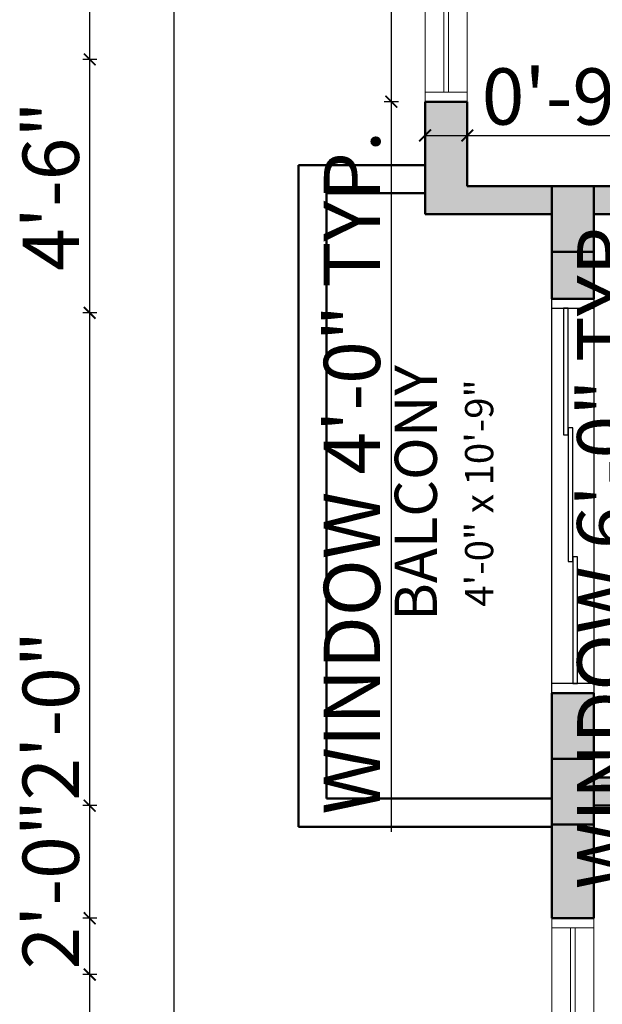
# Model space of a CAD drawing. Units: inches. Extents: x 375 to 1122, y 27 to 1069.
# Tile 72 of 155: x 385 to 509, y 667 to 877. Entities that reach past the tile are written whole.
import ezdxf

# ---------------------------------------------------------------- set-up
doc = ezdxf.new("R2010")
doc.units = ezdxf.units.IN
for name, color, linetype, lineweight in [('A-ANNO-DIMS', 2, 'Continuous', 18), ('A-AREA-IDEN', 7, 'Continuous', 18), ('A-COLS-PATT', 10, 'Continuous', 13), ('A-WALL-PATT', 252, 'Continuous', 13), ('Columns', 10, 'Continuous', 50), ('Doors', 150, 'Continuous', 25), ('Walls', 250, 'Continuous', 50), ('Windows', 122, 'Continuous', 18)]:
    doc.layers.add(name, color=color, linetype=linetype, lineweight=lineweight)
doc.styles.get("Standard").update_dxf_attribs({"font": 'arial.ttf'})
doc.dimstyles.new('ISO-25', dxfattribs={"dimtxt": 12, "dimasz": 2.5, "dimexe": 1.5, "dimexo": 1.5, "dimtad": 1, "dimdec": 1, "dimlunit": 3, "dimtxsty": 'Standard', "dimblk": 'ARCHTICK', "dimcen": 2.5, "dimadec": 0, "dimazin": 0, "dimtfac": 1, "dimtdec": 1, "dimtmove": 0, "dimatfit": 3, "dimfxl": 1.5, "dimfxlon": 1, "dimarcsym": 0})

# ---------------------------------------------------------------- blocks, each defined once
blk = doc.blocks.new('_ArchTick')
at = {"color": 0, "linetype": 'ByBlock', "const_width": 0.15}
blk.add_lwpolyline([(-0.5, -0.5), (0.5, 0.5)], dxfattribs=at)
blk = doc.blocks.new('*D28')
at = {"layer": 'A-ANNO-DIMS', "color": 0, "lineweight": -2, "transparency": 16777216}
for p, q in [((419.42, 982.53), (416.42, 982.53)), ((417.92, 982.53), (417.92, 187.53)), ((419.42, 187.53), (416.42, 187.53))]:
    blk.add_line(p, q, dxfattribs=at)
at = {"layer": 'Defpoints', "color": 0, "transparency": 16777216}
for p in [(444.51, 982.53), (417.92, 187.53), (444.51, 187.53)]:
    blk.add_point(p, dxfattribs=at)
at = {"layer": 'A-ANNO-DIMS', "color": 0, "lineweight": -2, "transparency": 16777216, "xscale": 2.5, "yscale": 2.5, "zscale": 2.5}
for p, rotation in [((417.92, 982.53), 90), ((417.92, 187.53), 270)]:
    blk.add_blockref('_ArchTick', p, dxfattribs=dict(at, rotation=rotation))
at = {"layer": 'A-ANNO-DIMS', "color": 0, "transparency": 16777216, "insert": (411.17, 585.03), "char_height": 12, "attachment_point": 5, "rotation": 90}
blk.add_mtext('66\'-3"', dxfattribs=at)
blk = doc.blocks.new('WINDOW-48IN')
for p, q in [((2, 5), (46, 5)), ((2, 4), (46, 4))]:
    blk.add_line(p, q)
blk.add_lwpolyline([(48, 0), (0, 0), (0, 9), (48, 9)], close=True)
for points in [[(2, 0), (2, 9)], [(46, 9), (46, 0)]]:
    blk.add_lwpolyline(points)
blk = doc.blocks.new('WINDOW-72IN')
for p, q in [((4, 70), (4, 2)), ((5, 70), (5, 2))]:
    blk.add_line(p, q)
blk.add_lwpolyline([(9, 0), (0, 0), (0, 72), (9, 72)], close=True)
for points in [[(0, 70), (9, 70)], [(9, 2), (0, 2)]]:
    blk.add_lwpolyline(points)
blk = doc.blocks.new('BALCONY-SLIDER-3P-84IN')
for points in [[(0, 84), (9, 84), (9, 0), (0, 0)], [(2.5, 55), (3.5, 55), (3.5, 82), (2.5, 82)], [(3.5, 28), (4.5, 28), (4.5, 56.5), (3.5, 56.5)], [(4.5, 2), (5.5, 2), (5.5, 29), (4.5, 29)]]:
    blk.add_lwpolyline(points, close=True)
for points in [[(0, 82), (9, 82)], [(9, 2), (0, 2)]]:
    blk.add_lwpolyline(points)
blk = doc.blocks.new('COLUMN-14X9IN')
blk.add_lwpolyline([(0, 0), (14, 0), (14, 9), (0, 9)], close=True)
blk = doc.blocks.new('*D47')
at = {"layer": 'A-ANNO-DIMS', "color": 0, "lineweight": -2, "transparency": 16777216}
for p, q in [((465.81, 907.53), (462.81, 907.53)), ((464.31, 907.53), (464.31, 859.53)), ((465.81, 859.53), (462.81, 859.53)), ((464.31, 859.53), (464.31, 703.93))]:
    blk.add_line(p, q, dxfattribs=at)
at = {"layer": 'Defpoints', "color": 0, "transparency": 16777216}
for p in [(471.51, 907.53), (464.31, 859.53), (471.51, 859.53)]:
    blk.add_point(p, dxfattribs=at)
at = {"layer": 'A-ANNO-DIMS', "color": 0, "lineweight": -2, "transparency": 16777216, "xscale": 2.5, "yscale": 2.5, "zscale": 2.5}
for p, rotation in [((464.31, 907.53), 90), ((464.31, 859.53), 270)]:
    blk.add_blockref('_ArchTick', p, dxfattribs=dict(at, rotation=rotation))
at = {"layer": 'A-ANNO-DIMS', "color": 0, "transparency": 16777216, "insert": (457.47, 780.48), "char_height": 12, "attachment_point": 5, "rotation": 90}
blk.add_mtext('WINDOW 4\'-0" TYP.', dxfattribs=at)
blk = doc.blocks.new('*D48')
at = {"layer": 'A-ANNO-DIMS', "color": 0, "lineweight": -2, "transparency": 16777216}
for p, q in [((471.51, 853.83), (471.51, 850.83)), ((471.51, 852.33), (480.51, 852.33)), ((480.51, 853.83), (480.51, 850.83)), ((480.51, 852.33), (557.4, 852.33))]:
    blk.add_line(p, q, dxfattribs=at)
at = {"layer": 'Defpoints', "color": 0, "transparency": 16777216}
for p in [(471.51, 859.53), (480.51, 859.53), (480.51, 852.33)]:
    blk.add_point(p, dxfattribs=at)
at = {"layer": 'A-ANNO-DIMS', "color": 0, "lineweight": -2, "transparency": 16777216, "xscale": 2.5, "yscale": 2.5, "zscale": 2.5, "rotation": 180}
blk.add_blockref('_ArchTick', (471.51, 852.33), dxfattribs=at)
at = {"layer": 'A-ANNO-DIMS', "color": 0, "lineweight": -2, "transparency": 16777216, "xscale": 2.5, "yscale": 2.5, "zscale": 2.5}
blk.add_blockref('_ArchTick', (480.51, 852.33), dxfattribs=at)
at = {"layer": 'A-ANNO-DIMS', "color": 0, "transparency": 16777216, "insert": (520.21, 859.08), "char_height": 12, "attachment_point": 5}
blk.add_mtext('0\'-9" TYP.', dxfattribs=at)
blk = doc.blocks.new('*D69')
at = {"layer": 'A-ANNO-DIMS', "color": 0, "lineweight": -2, "transparency": 16777216}
for p, q in [((518.31, 685.53), (518.31, 841.13)), ((516.81, 685.53), (519.81, 685.53)), ((518.31, 613.53), (518.31, 685.53)), ((516.81, 613.53), (519.81, 613.53))]:
    blk.add_line(p, q, dxfattribs=at)
at = {"layer": 'Defpoints', "color": 0, "transparency": 16777216}
for p in [(507.51, 685.53), (518.31, 685.53), (507.51, 613.53)]:
    blk.add_point(p, dxfattribs=at)
at = {"layer": 'A-ANNO-DIMS', "color": 0, "lineweight": -2, "transparency": 16777216, "xscale": 2.5, "yscale": 2.5, "zscale": 2.5}
for p, rotation in [((518.31, 685.53), 90), ((518.31, 613.53), 270)]:
    blk.add_blockref('_ArchTick', p, dxfattribs=dict(at, rotation=rotation))
at = {"layer": 'A-ANNO-DIMS', "color": 0, "transparency": 16777216, "insert": (511.47, 764.58), "char_height": 12, "attachment_point": 5, "rotation": 90}
blk.add_mtext('WINDOW 6\'-0" TYP.', dxfattribs=at)
blk = doc.blocks.new('*D82')
at = {"layer": 'A-ANNO-DIMS', "color": 0, "lineweight": -2, "transparency": 16777216}
for p, q in [((401.51, 1009.53), (398.51, 1009.53)), ((400.01, 160.53), (400.01, 1009.53)), ((401.51, 160.53), (398.51, 160.53))]:
    blk.add_line(p, q, dxfattribs=at)
at = {"layer": 'Defpoints', "color": 0, "transparency": 16777216}
for p in [(400.01, 1009.53), (630.53, 1009.53), (630.53, 160.53)]:
    blk.add_point(p, dxfattribs=at)
at = {"layer": 'A-ANNO-DIMS', "color": 0, "lineweight": -2, "transparency": 16777216, "xscale": 2.5, "yscale": 2.5, "zscale": 2.5}
for p, rotation in [((400.01, 1009.53), 90), ((400.01, 160.53), 270)]:
    blk.add_blockref('_ArchTick', p, dxfattribs=dict(at, rotation=rotation))
at = {"layer": 'A-ANNO-DIMS', "color": 0, "transparency": 16777216, "insert": (393.26, 585.03), "char_height": 12, "attachment_point": 5, "rotation": 90}
blk.add_mtext('70\'-9"', dxfattribs=at)
blk = doc.blocks.new('*D85')
at = {"layer": 'A-ANNO-DIMS', "color": 0, "lineweight": -2, "transparency": 16777216}
for p, q in [((401.51, 868.53), (398.51, 868.53)), ((400.01, 814.53), (400.01, 868.53)), ((401.51, 814.53), (398.51, 814.53))]:
    blk.add_line(p, q, dxfattribs=at)
at = {"layer": 'Defpoints', "color": 0, "transparency": 16777216}
for p in [(400.01, 868.53), (845.01, 868.53), (845.01, 814.53)]:
    blk.add_point(p, dxfattribs=at)
at = {"layer": 'A-ANNO-DIMS', "color": 0, "lineweight": -2, "transparency": 16777216, "xscale": 2.5, "yscale": 2.5, "zscale": 2.5}
for p, rotation in [((400.01, 868.53), 90), ((400.01, 814.53), 270)]:
    blk.add_blockref('_ArchTick', p, dxfattribs=dict(at, rotation=rotation))
at = {"layer": 'A-ANNO-DIMS', "color": 0, "transparency": 16777216, "insert": (393.26, 841.53), "char_height": 12, "attachment_point": 5, "rotation": 90}
blk.add_mtext('4\'-6"', dxfattribs=at)
blk = doc.blocks.new('*D93')
at = {"layer": 'A-ANNO-DIMS', "color": 0, "lineweight": -2, "transparency": 16777216}
for p, q in [((400.01, 673.53), (400.01, 709.38)), ((401.51, 673.53), (398.51, 673.53)), ((400.01, 649.53), (400.01, 673.53)), ((401.51, 649.53), (398.51, 649.53))]:
    blk.add_line(p, q, dxfattribs=at)
at = {"layer": 'Defpoints', "color": 0, "transparency": 16777216}
for p in [(400.01, 673.53), (663.51, 673.53), (663.51, 649.53)]:
    blk.add_point(p, dxfattribs=at)
at = {"layer": 'A-ANNO-DIMS', "color": 0, "lineweight": -2, "transparency": 16777216, "xscale": 2.5, "yscale": 2.5, "zscale": 2.5}
for p, rotation in [((400.01, 673.53), 90), ((400.01, 649.53), 270)]:
    blk.add_blockref('_ArchTick', p, dxfattribs=dict(at, rotation=rotation))
at = {"layer": 'A-ANNO-DIMS', "color": 0, "transparency": 16777216, "insert": (393.26, 692.7), "char_height": 12, "attachment_point": 5, "rotation": 90}
blk.add_mtext('2\'-0"', dxfattribs=at)
blk = doc.blocks.new('*D95')
at = {"layer": 'A-ANNO-DIMS', "color": 0, "lineweight": -2, "transparency": 16777216}
for p, q in [((400.01, 709.53), (400.01, 745.38)), ((401.51, 709.53), (398.51, 709.53)), ((400.01, 685.53), (400.01, 709.53)), ((401.51, 685.53), (398.51, 685.53))]:
    blk.add_line(p, q, dxfattribs=at)
at = {"layer": 'Defpoints', "color": 0, "transparency": 16777216}
for p in [(400.01, 709.53), (507.51, 709.53), (507.51, 685.53)]:
    blk.add_point(p, dxfattribs=at)
at = {"layer": 'A-ANNO-DIMS', "color": 0, "lineweight": -2, "transparency": 16777216, "xscale": 2.5, "yscale": 2.5, "zscale": 2.5}
for p, rotation in [((400.01, 709.53), 90), ((400.01, 685.53), 270)]:
    blk.add_blockref('_ArchTick', p, dxfattribs=dict(at, rotation=rotation))
at = {"layer": 'A-ANNO-DIMS', "color": 0, "transparency": 16777216, "insert": (393.26, 728.7), "char_height": 12, "attachment_point": 5, "rotation": 90}
blk.add_mtext('2\'-0"', dxfattribs=at)

msp = doc.modelspace()

# ---------------------------------------------------------------- hatches: boundary and pattern name
at = {"layer": 'A-COLS-PATT'}
h = msp.add_hatch(color=256, dxfattribs=at)
h.dxf.hatch_style = 1
h.paths.add_polyline_path([(512.51, 982.53), (498.51, 982.53), (498.51, 973.53), (512.51, 973.53)])
h.paths.add_polyline_path([(666.51, 982.53), (652.51, 982.53), (652.51, 973.53), (666.51, 973.53)])
h.paths.add_polyline_path([(802.01, 982.53), (788.01, 982.53), (788.01, 973.53), (802.01, 973.53)])
h.paths.add_polyline_path([(932.01, 982.53), (918.01, 982.53), (918.01, 973.53), (932.01, 973.53)])
h.paths.add_polyline_path([(507.51, 841.53), (498.51, 841.53), (498.51, 827.53), (507.51, 827.53)])
h.paths.add_polyline_path([(666.51, 844.53), (652.51, 844.53), (652.51, 835.53), (666.51, 835.53)])
h.paths.add_polyline_path([(802.01, 814.53), (788.01, 814.53), (788.01, 805.53), (802.01, 805.53)])
h.paths.add_polyline_path([(932.01, 814.53), (918.01, 814.53), (918.01, 805.53), (932.01, 805.53)])
h.paths.add_polyline_path([(507.51, 719.53), (498.51, 719.53), (498.51, 705.53), (507.51, 705.53)])
h.paths.add_polyline_path([(731.01, 676.53), (722.01, 676.53), (722.01, 662.53), (731.01, 662.53)])
h.paths.add_polyline_path([(802.01, 676.53), (788.01, 676.53), (788.01, 667.53), (802.01, 667.53)])
h.paths.add_polyline_path([(932.01, 676.53), (918.01, 676.53), (918.01, 667.53), (932.01, 667.53)])
h.paths.add_polyline_path([(932.01, 583.53), (918.01, 583.53), (918.01, 574.53), (932.01, 574.53)])
h.paths.add_polyline_path([(868.01, 583.53), (854.01, 583.53), (854.01, 574.53), (868.01, 574.53)])
h.paths.add_polyline_path([(868.01, 502.53), (854.01, 502.53), (854.01, 493.53), (868.01, 493.53)])
h.paths.add_polyline_path([(932.01, 502.53), (918.01, 502.53), (918.01, 493.53), (932.01, 493.53)])
h.paths.add_polyline_path([(672.51, 592.03), (663.51, 592.03), (663.51, 578.03), (672.51, 578.03)])
h.paths.add_polyline_path([(512.51, 589.53), (498.51, 589.53), (498.51, 580.53), (512.51, 580.53)])
h.paths.add_polyline_path([(507.51, 464.53), (498.51, 464.53), (498.51, 450.53), (507.51, 450.53)])
h.paths.add_polyline_path([(731.01, 507.53), (722.01, 507.53), (722.01, 493.53), (731.01, 493.53)])
h.paths.add_polyline_path([(802.01, 502.53), (788.01, 502.53), (788.01, 493.53), (802.01, 493.53)])
h.paths.add_polyline_path([(507.51, 342.53), (498.51, 342.53), (498.51, 328.53), (507.51, 328.53)])
h.paths.add_polyline_path([(512.51, 196.53), (498.51, 196.53), (498.51, 187.53), (512.51, 187.53)])
h.paths.add_polyline_path([(666.51, 334.53), (652.51, 334.53), (652.51, 325.53), (666.51, 325.53)])
h.paths.add_polyline_path([(666.51, 196.53), (652.51, 196.53), (652.51, 187.53), (666.51, 187.53)])
h.paths.add_polyline_path([(805.01, 196.53), (791.01, 196.53), (791.01, 187.53), (805.01, 187.53)])
h.paths.add_polyline_path([(932.01, 196.53), (918.01, 196.53), (918.01, 187.53), (932.01, 187.53)])
h.paths.add_polyline_path([(932.01, 334.53), (918.01, 334.53), (918.01, 325.53), (932.01, 325.53)])
h.paths.add_polyline_path([(805.01, 334.53), (791.01, 334.53), (791.01, 325.53), (805.01, 325.53)])
at = {"layer": 'A-WALL-PATT'}
h = msp.add_hatch(color=256, dxfattribs=at)
h.dxf.hatch_style = 1
h.paths.add_polyline_path([(962.01, 388.53), (989.01, 388.53), (989.01, 394.53), (962.01, 394.53), (932.01, 394.53), (932.01, 397.53), (923.01, 397.53), (923.01, 394.53), (842.01, 394.53), (842.01, 334.53), (839.51, 334.53), (839.51, 328.53), (854.01, 328.53), (854.01, 334.53), (848.01, 334.53), (848.01, 388.53), (953.01, 388.53), (953.01, 356.08), (962.01, 356.08), (962.01, 358.55), (989.01, 358.55), (989.01, 364.55), (962.01, 364.55)])
h.paths.add_polyline_path([(989.01, 502.53), (932.01, 502.53), (932.01, 583.53), (932.01, 593.53), (923.01, 593.53), (923.01, 583.53), (854.01, 583.53), (854.01, 556.53), (863.01, 556.53), (863.01, 574.53), (923.01, 574.53), (923.01, 502.53), (863.01, 502.53), (863.01, 520.53), (854.01, 520.53), (854.01, 502.53), (773.01, 502.53), (773.01, 493.53), (788.01, 493.53), (788.01, 402.03), (722.01, 402.03), (722.01, 373.53), (728.01, 373.53), (728.01, 396.03), (788.01, 396.03), (788.01, 373.53), (794.01, 373.53), (794.01, 430.53), (814.01, 430.53), (814.01, 436.53), (794.01, 436.53), (794.01, 493.53), (923.01, 493.53), (923.01, 487.53), (932.01, 487.53), (932.01, 493.53), (983.01, 493.53), (983.01, 473.53), (989.01, 473.53)])
h.paths.add_polyline_path([(797.01, 325.53), (805.01, 325.53), (805.01, 328.53), (807.51, 328.53), (807.51, 334.53), (791.01, 334.53), (791.01, 226.53), (770.76, 226.53), (770.76, 217.53), (791.01, 217.53), (791.01, 187.53), (855.01, 187.53), (855.01, 196.53), (797.01, 196.53)])
h.paths.add_polyline_path([(989.01, 238.53), (962.01, 238.53), (962.01, 256.42), (953.01, 256.42), (953.01, 229.53), (980.01, 229.53), (980.01, 196.53), (915.01, 196.53), (915.01, 187.53), (989.01, 187.53)])
h.paths.add_polyline_path([(962.01, 334.53), (884.01, 334.53), (884.01, 328.53), (918.01, 328.53), (918.01, 325.53), (932.01, 325.53), (932.01, 328.53), (953.01, 328.53), (953.01, 304.42), (962.01, 304.42)])
h.paths.add_polyline_path([(606.51, 283.53), (609.51, 283.53), (609.51, 289.53), (600.51, 289.53), (600.51, 196.53), (578.51, 196.53), (578.51, 187.53), (606.51, 187.53), (606.51, 196.53)])
h.paths.add_polyline_path([(666.51, 292.53), (660.51, 292.53), (660.51, 289.53), (633.51, 289.53), (633.51, 283.53), (660.51, 283.53), (660.51, 196.53), (628.01, 196.53), (628.01, 187.53), (630.53, 187.53), (630.53, 160.53), (636.53, 160.53), (636.53, 187.53), (660.51, 187.53), (660.51, 160.53), (666.51, 160.53), (666.51, 217.53), (686.76, 217.53), (686.76, 226.53), (666.51, 226.53)])
h.paths.add_polyline_path([(480.51, 256.42), (471.51, 256.42), (471.51, 238.53), (444.51, 238.53), (444.51, 187.53), (518.51, 187.53), (518.51, 196.53), (453.51, 196.53), (453.51, 229.53), (480.51, 229.53)])
h.paths.add_polyline_path([(480.51, 328.53), (652.51, 328.53), (652.51, 325.53), (660.51, 325.53), (660.51, 322.53), (666.51, 322.53), (666.51, 334.53), (507.51, 334.53), (507.51, 360.53), (498.51, 360.53), (498.51, 334.53), (471.51, 334.53), (471.51, 304.42), (480.51, 304.42)])
h.paths.add_polyline_path([(507.51, 484.53), (498.51, 484.53), (498.51, 444.53), (507.51, 444.53), (507.51, 454.53), (621.51, 454.53), (621.51, 460.53), (507.51, 460.53)])
h.paths.add_polyline_path([(672.51, 604.53), (683.26, 604.53), (683.26, 613.53), (669.51, 613.53), (669.51, 649.53), (663.51, 649.53), (663.51, 589.53), (507.51, 589.53), (507.51, 613.53), (498.51, 613.53), (498.51, 556.53), (507.51, 556.53), (507.51, 580.53), (663.51, 580.53), (663.51, 520.53), (669.51, 520.53), (669.51, 556.53), (683.26, 556.53), (683.26, 565.53), (672.51, 565.53)])
h.paths.add_polyline_path([(731.01, 667.53), (734.01, 667.53), (734.01, 676.53), (728.01, 676.53), (728.01, 715.53), (657.51, 715.53), (657.51, 709.53), (663.51, 709.53), (663.51, 673.53), (669.51, 673.53), (669.51, 709.53), (722.01, 709.53), (722.01, 613.53), (704.76, 613.53), (704.76, 604.53), (722.01, 604.53), (722.01, 565.53), (704.76, 565.53), (704.76, 556.53), (722.01, 556.53), (722.01, 502.53), (722.01, 460.53), (669.51, 460.53), (669.51, 496.53), (663.51, 496.53), (663.51, 460.53), (657.51, 460.53), (657.51, 454.53), (728.01, 454.53), (728.01, 493.53), (734.01, 493.53), (734.01, 502.53), (731.01, 502.53)])
h.paths.add_polyline_path([(986.01, 718.53), (959.01, 718.53), (959.01, 727.53), (950.01, 727.53), (950.01, 709.53), (977.01, 709.53), (977.01, 676.53), (794.01, 676.53), (794.01, 805.53), (802.01, 805.53), (802.01, 808.53), (804.51, 808.53), (804.51, 814.53), (788.01, 814.53), (788.01, 774.03), (728.01, 774.03), (728.01, 796.53), (722.01, 796.53), (722.01, 768.03), (788.01, 768.03), (788.01, 676.53), (773.01, 676.53), (773.01, 667.53), (923.01, 667.53), (923.01, 657.53), (932.01, 657.53), (932.01, 667.53), (986.01, 667.53)])
h.paths.add_polyline_path([(621.51, 715.53), (507.51, 715.53), (507.51, 733.53), (498.51, 733.53), (498.51, 715.53), (498.51, 685.53), (507.51, 685.53), (507.51, 709.53), (621.51, 709.53)])
h.paths.add_polyline_path([(666.51, 847.03), (660.51, 847.03), (660.51, 844.53), (652.51, 844.53), (652.51, 841.53), (480.51, 841.53), (480.51, 859.53), (471.51, 859.53), (471.51, 835.53), (498.51, 835.53), (498.51, 817.53), (507.51, 817.53), (507.51, 835.53), (666.51, 835.53)])
h.paths.add_polyline_path([(480.51, 940.53), (453.51, 940.53), (453.51, 973.53), (518.51, 973.53), (518.51, 982.53), (444.51, 982.53), (444.51, 931.53), (471.51, 931.53), (471.51, 907.53), (480.51, 907.53)])
h.paths.add_polyline_path([(606.51, 982.53), (578.51, 982.53), (578.51, 973.53), (600.51, 973.53), (600.51, 880.53), (609.51, 880.53), (609.51, 886.53), (606.51, 886.53)])
h.paths.add_polyline_path([(666.51, 943.53), (686.76, 943.53), (686.76, 952.53), (666.51, 952.53), (666.51, 1009.53), (660.51, 1009.53), (660.51, 982.53), (636.53, 982.53), (636.53, 1009.53), (630.53, 1009.53), (630.53, 982.53), (628.01, 982.53), (628.01, 973.53), (660.51, 973.53), (660.51, 886.53), (633.51, 886.53), (633.51, 880.53), (660.51, 880.53), (660.51, 877.03), (666.51, 877.03)])
h.paths.add_polyline_path([(986.01, 874.53), (932.01, 874.53), (932.01, 877.53), (923.01, 877.53), (923.01, 874.53), (788.01, 874.53), (788.01, 868.53), (788.01, 844.53), (794.01, 844.53), (794.01, 868.53), (839.01, 868.53), (839.01, 814.53), (836.51, 814.53), (836.51, 808.53), (851.01, 808.53), (851.01, 814.53), (845.01, 814.53), (845.01, 868.53), (986.01, 868.53)])
h.paths.add_polyline_path([(959.01, 838.55), (986.01, 838.55), (986.01, 844.55), (959.01, 844.55), (959.01, 847.03), (950.01, 847.03), (950.01, 814.53), (881.01, 814.53), (881.01, 808.53), (918.01, 808.53), (918.01, 805.53), (932.01, 805.53), (932.01, 808.53), (950.01, 808.53), (950.01, 793.53), (959.01, 793.53)])
h.paths.add_polyline_path([(986.01, 982.53), (899.01, 982.53), (899.01, 973.53), (923.01, 973.53), (923.01, 967.53), (932.01, 967.53), (932.01, 973.53), (980.01, 973.53), (980.01, 953.53), (986.01, 953.53)])
h.paths.add_polyline_path([(851.01, 982.53), (788.01, 982.53), (788.01, 952.53), (770.76, 952.53), (770.76, 943.53), (788.01, 943.53), (788.01, 910.53), (814.01, 910.53), (814.01, 916.53), (794.01, 916.53), (794.01, 973.53), (851.01, 973.53)])

# ---------------------------------------------------------------- linework, layer by layer
at = {"layer": 'Walls'}
for p, q in [((480.51, 859.53), (471.51, 859.53)), ((471.51, 859.53), (471.51, 835.53)), ((480.51, 859.53), (480.51, 841.53)), ((444.51, 846.03), (471.51, 846.03)), ((444.51, 846.03), (444.51, 705.03)), ((480.51, 841.53), (652.51, 841.53)), ((450.51, 840.03), (471.51, 840.03)), ((450.51, 840.03), (450.51, 711.03)), ((471.51, 835.53), (498.51, 835.53)), ((498.51, 835.53), (498.51, 817.53)), ((507.51, 835.53), (507.51, 817.53)), ((507.51, 835.53), (666.51, 835.53)), ((507.51, 817.53), (498.51, 817.53)), ((507.51, 733.53), (498.51, 733.53)), ((498.51, 733.53), (498.51, 715.53)), ((507.51, 733.53), (507.51, 715.53)), ((498.51, 685.53), (498.51, 715.53)), ((507.51, 715.53), (621.51, 715.53)), ((450.51, 711.03), (498.51, 711.03)), ((507.51, 709.53), (621.51, 709.53)), ((507.51, 685.53), (507.51, 709.53)), ((444.51, 705.03), (498.51, 705.03)), ((507.51, 685.53), (498.51, 685.53))]:
    msp.add_line(p, q, dxfattribs=at)

# ---------------------------------------------------------------- block references
at = {"layer": 'Columns', "extrusion": (0, 0, -1), "zscale": -1, "rotation": 90}
for p in [(-498.51, 827.53), (-498.51, 705.53)]:
    msp.add_blockref('COLUMN-14X9IN', p, dxfattribs=at)
at = {"layer": 'Doors'}
msp.add_blockref('BALCONY-SLIDER-3P-84IN', (498.51, 733.53), dxfattribs=at)
at = {"layer": 'Windows', "rotation": 270}
msp.add_blockref('WINDOW-48IN', (471.51, 907.53), dxfattribs=at)
at = {"layer": 'Windows'}
msp.add_blockref('WINDOW-72IN', (498.51, 613.53), dxfattribs=at)

# ---------------------------------------------------------------- texts
at = {"layer": 'A-AREA-IDEN', "insert": (465.03, 809.21), "char_height": 12, "attachment_point": 3, "rotation": 90}
msp.add_mtext_dynamic_manual_height_columns('\\pxqc;{\\fArial|b1|i0|c0|p34;\\H0.75x;BALCONY\\H1.33333x;\\P\\fArial|b0|i0|c0|p34;\\H0.5x;4\'-0" x 10\'-9"}', width=66.1169, gutter_width=12.5, heights=[0], dxfattribs=at)

# ---------------------------------------------------------------- dimensions: what is measured, and where the dimension line sits
at = {"layer": 'A-ANNO-DIMS'}
for base, p1, p2, override, picture, middle in [((400.01, 1009.53), (630.53, 160.53), (630.53, 1009.53), {"dimdec": 1, "dimlfac": 1, "dimrnd": 0, "dimzin": 1, "dimdsep": 46, "dimlunit": 4, "dimfrac": 2}, '*D82', (393.26, 585.03)), ((417.92, 187.53), (444.51, 982.53), (444.51, 187.53), {"dimclrd": 0, "dimclre": 0, "dimclrt": 0}, '*D28', (411.17, 585.03)), ((400.01, 868.53), (845.01, 814.53), (845.01, 868.53), {"dimdec": 1, "dimlfac": 1, "dimrnd": 0, "dimzin": 1, "dimdsep": 46, "dimlunit": 4, "dimfrac": 2}, '*D85', (393.26, 841.53)), ((400.01, 709.53), (507.51, 685.53), (507.51, 709.53), {"dimdec": 1, "dimlfac": 1, "dimrnd": 0, "dimzin": 1, "dimdsep": 46, "dimlunit": 4, "dimfrac": 2}, '*D95', (393.26, 728.7)), ((400.01, 673.53), (663.51, 649.53), (663.51, 673.53), {"dimdec": 1, "dimlfac": 1, "dimrnd": 0, "dimzin": 1, "dimdsep": 46, "dimlunit": 4, "dimfrac": 2}, '*D93', (393.26, 692.7))]:
    dim = msp.add_linear_dim(base=base, p1=p1, p2=p2, angle=90, dimstyle='ISO-25', override=override, dxfattribs=at)
    dim.commit()
    dim.dimension.update_dxf_attribs({"geometry": picture, "text_midpoint": middle})
for base, p1, p2, angle, picture, middle in [((464.31, 859.53), (471.51, 907.53), (471.51, 859.53), 270, '*D47', (457.47, 780.48)), ((518.31, 685.53), (507.51, 613.53), (507.51, 685.53), 90, '*D69', (511.47, 764.58))]:
    dim = msp.add_linear_dim(base=base, p1=p1, p2=p2, angle=angle, text='WINDOW <> TYP.', dimstyle='ISO-25', override={"dimdec": 1, "dimlfac": 1, "dimrnd": 0, "dimzin": 1, "dimdsep": 46, "dimlunit": 4, "dimfrac": 2}, dxfattribs=at)
    dim.commit()
    dim.dimension.update_dxf_attribs({"geometry": picture, "text_midpoint": middle})
dim = msp.add_linear_dim(base=(480.51, 852.33), p1=(471.51, 859.53), p2=(480.51, 859.53), text='<> TYP.', dimstyle='ISO-25', override={"dimdec": 1, "dimlfac": 1, "dimrnd": 0, "dimzin": 1, "dimdsep": 46, "dimlunit": 4, "dimfrac": 2}, dxfattribs=at)
dim.commit()
dim.dimension.update_dxf_attribs({"geometry": '*D48', "text_midpoint": (520.21, 859.08)})

doc.saveas('drawing.dxf')
